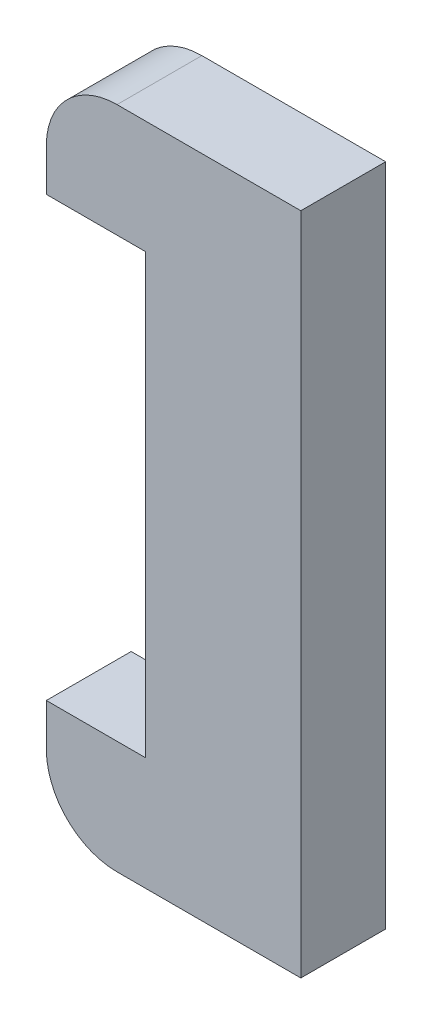
from build123d import *

# Parameters (mm, degrees)
GIB_BODY_EXTRUDE_12MM_DEPTH = 6


with BuildPart() as part:
    # Gib Profile Sketch → Gib Body Extrude 12mm (new, symmetric)
    with BuildSketch(Plane.XY):
        with BuildLine():
            Line((-26, 30.177777778), (0, 30.177777778))
            Line((0, 30.177777778), (0, -63.822222222))
            Line((0, -63.822222222), (-26, -63.822222222))
            ThreePointArc((-26, -63.822222222), (-33.071067812, -60.893290034), (-36, -53.822222222))
            Line((-36, -53.822222222), (-36, -47.822222222))
            Line((-36, -47.822222222), (-22, -47.822222222))
            Line((-22, -47.822222222), (-22, 14.177777778))
            Line((-22, 14.177777778), (-36, 14.177777778))
            Line((-36, 14.177777778), (-36, 20.177777778))
            ThreePointArc((-36, 20.177777778), (-33.071067812, 27.24884559), (-26, 30.177777778))
        make_face()
    extrude(amount=GIB_BODY_EXTRUDE_12MM_DEPTH, both=True)


solid = part.part
